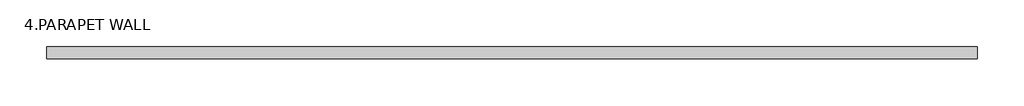
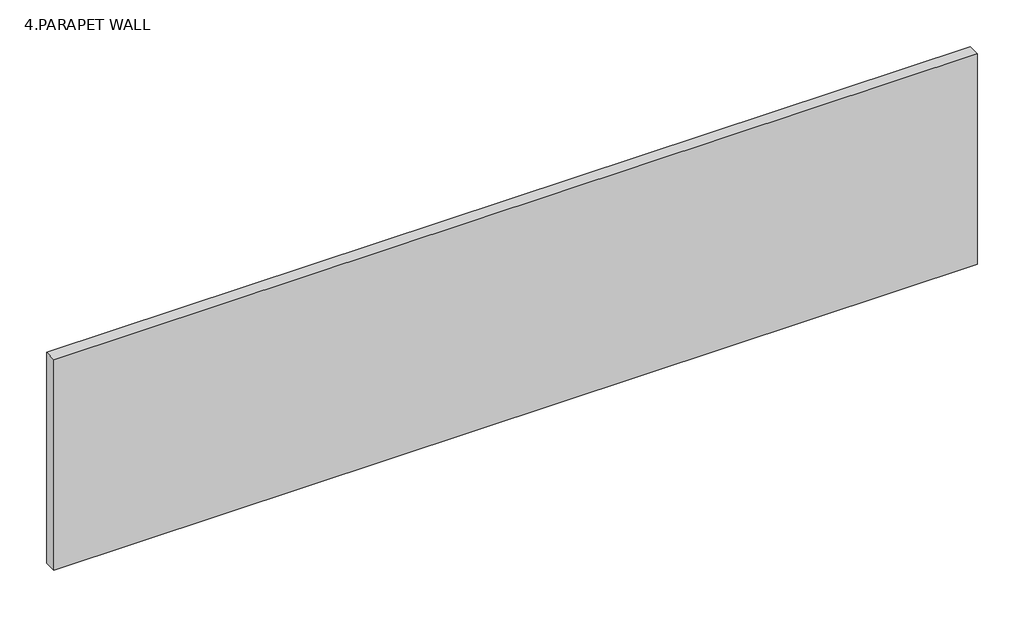
# One storey: 1 plate.
"""IFC4 building model written with IfcOpenShell, lengths in millimetres."""

from ifc_helpers import new_model, si_unit, origin, place, context, project, spatial, transform, mapped, element, save
from components import system_panel_glazed_7d5859e6

model = new_model("IFC4")

# Units and contexts
model_context = context("Model", 3, world=origin())
ifc_project = project(units=[si_unit("LENGTHUNIT", "METRE", prefix="MILLI")], contexts=[model_context])

# Site, building, storey
site = spatial("IfcSite", under=ifc_project)
building = spatial("IfcBuilding", under=site)
storey = spatial("IfcBuildingStorey", under=building, Name="4.PARAPET WALL", Elevation=7924.8)

# Plate
placement = place(None, origin())
system_panel_glazed_shape = system_panel_glazed_7d5859e6(model_context)
element("IfcPlate", 1, ObjectType="System Panel : Glazed", at=placement, inside=storey, context=model_context, shape_type="MappedRepresentation", body=[
    mapped(system_panel_glazed_shape, transform((-1429.2657257, 2.5160289, 6307.1112081), x_axis=(1.0, 0.0, 0.0), y_axis=(0.0, 1.0, 0.0), z_axis=(0.0, 0.0, 1.0))),
])

save(model, "model.ifc")

# Revit data of these elements
# Type "System Panel : Glazed"
#   Construction Type Id = "GSP4R"
#   Analytic Construction = "1/8 in Pilkington single glazing"
#   Visual Light Transmittance = 0.9
#   Solar Heat Gain Coefficient = 0.86
#   Heat Transfer Coefficient (U) = 1.18115 BTU/(h·ft²·°F)
#   Define Thermal Properties by = 1
# Element 1 (IfcPlate, "System Panel : Glazed")
#   Phase Created = New Construction
#   Materials on its faces: "Glass"
# Materials
#   "Glass": class "Glass", colour RGB 0 128 192, transparency 0.75, Description = "Soda Lime Glass", Cost = 0
